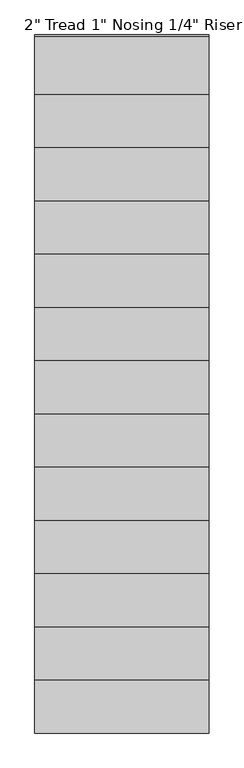
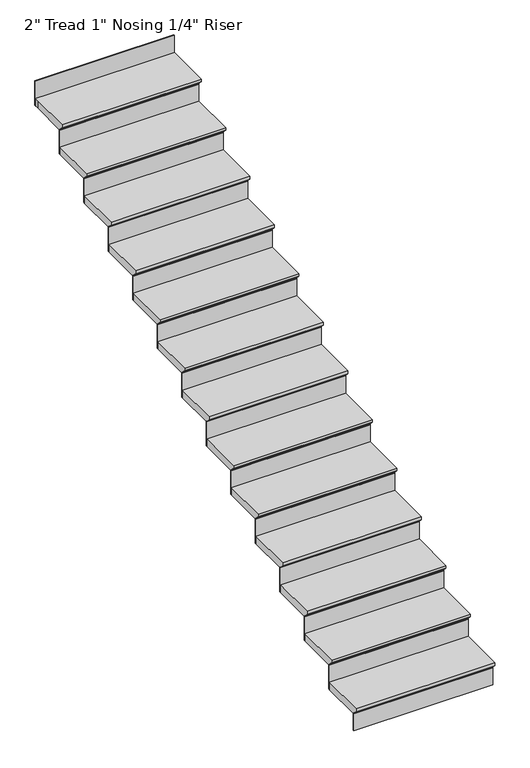
"""IFC4 building model written with IfcOpenShell, lengths in millimetres: stair flight geometry."""

from ifc_helpers import new_model, si_unit, origin, place, context, project, spatial, faceted_brep, source, transform, mapped, element, save


def stair_flight_c80e62dd(model_context):
    return source(origin(), model_context, "Body", "Brep", [
        faceted_brep([(-2703.0415084, -23154.3851539, 37576.9005799), (-2703.0415084, -23154.3851539, 37595.9505799), (-3617.4415084, -23154.3851539, 37595.9505799), (-3617.4415084, -23154.3851539, 37576.9005799), (-2703.0415084, -23128.9851539, 37551.5005799), (-3617.4415084, -23128.9851539, 37551.5005799), (-2703.0415084, -22849.5851539, 37595.9505799), (-3617.4415084, -22849.5851539, 37595.9505799), (-3617.4415084, -23128.9851539, 37545.1505799), (-3617.4415084, -22849.5851539, 37545.1505799), (-2703.0415084, -22849.5851539, 37545.1505799), (-2703.0415084, -23128.9851539, 37545.1505799)], [[[0, 1, 2, 3]], [[4, 0, 3, 5]], [[2, 1, 6, 7]], [[8, 9, 10, 11]], [[2, 7, 9, 8, 5, 3]], [[8, 11, 4, 5]], [[6, 1, 0, 4, 11, 10]], [[7, 6, 10, 9]]]),
        faceted_brep([(-2703.0415084, -23128.9851539, 37545.1505799), (-2703.0415084, -23128.9851539, 37426.6172466), (-2703.0415084, -23122.6351539, 37426.6172466), (-2703.0415084, -23122.6351539, 37545.1505799), (-3617.4415084, -23128.9851539, 37545.1505799), (-3617.4415084, -23122.6351539, 37545.1505799), (-3617.4415084, -23122.6351539, 37426.6172466), (-3617.4415084, -23128.9851539, 37426.6172466)], [[[0, 1, 2, 3]], [[4, 5, 6, 7]], [[1, 0, 4, 7]], [[2, 1, 7, 6]], [[3, 2, 6, 5]], [[0, 3, 5, 4]]]),
        faceted_brep([(-2703.0415084, -22849.5851539, 37714.4839133), (-2703.0415084, -22849.5851539, 37545.1505799), (-2703.0415084, -22843.2351539, 37545.1505799), (-2703.0415084, -22843.2351539, 37714.4839133), (-3617.4415084, -22849.5851539, 37714.4839133), (-3617.4415084, -22843.2351539, 37714.4839133), (-3617.4415084, -22843.2351539, 37545.1505799), (-3617.4415084, -22849.5851539, 37545.1505799)], [[[0, 1, 2, 3]], [[4, 5, 6, 7]], [[1, 0, 4, 7]], [[2, 1, 7, 6]], [[3, 2, 6, 5]], [[0, 3, 5, 4]]]),
        faceted_brep([(-3617.4415084, -22874.9851539, 37765.2839133), (-2703.0415084, -22874.9851539, 37765.2839133), (-2703.0415084, -22570.1851539, 37765.2839133), (-3617.4415084, -22570.1851539, 37765.2839133), (-3617.4415084, -22849.5851539, 37714.4839133), (-3617.4415084, -22570.1851539, 37714.4839133), (-2703.0415084, -22570.1851539, 37714.4839133), (-2703.0415084, -22849.5851539, 37714.4839133), (-3617.4415084, -22849.5851539, 37720.8339133), (-3617.4415084, -22874.9851539, 37746.2339133), (-2703.0415084, -22849.5851539, 37720.8339133), (-2703.0415084, -22874.9851539, 37746.2339133)], [[[0, 1, 2, 3]], [[4, 5, 6, 7]], [[0, 3, 5, 4, 8, 9]], [[4, 7, 10, 8]], [[2, 1, 11, 10, 7, 6]], [[3, 2, 6, 5]], [[11, 1, 0, 9]], [[10, 11, 9, 8]]]),
        faceted_brep([(-2703.0415084, -22570.1851539, 37883.8172466), (-2703.0415084, -22570.1851539, 37714.4839133), (-2703.0415084, -22563.8351539, 37714.4839133), (-2703.0415084, -22563.8351539, 37883.8172466), (-3617.4415084, -22570.1851539, 37883.8172466), (-3617.4415084, -22563.8351539, 37883.8172466), (-3617.4415084, -22563.8351539, 37714.4839133), (-3617.4415084, -22570.1851539, 37714.4839133)], [[[0, 1, 2, 3]], [[4, 5, 6, 7]], [[1, 0, 4, 7]], [[2, 1, 7, 6]], [[3, 2, 6, 5]], [[0, 3, 5, 4]]]),
        faceted_brep([(-3617.4415084, -22595.5851539, 37934.6172466), (-2703.0415084, -22595.5851539, 37934.6172466), (-2703.0415084, -22290.7851539, 37934.6172466), (-3617.4415084, -22290.7851539, 37934.6172466), (-3617.4415084, -22570.1851539, 37883.8172466), (-3617.4415084, -22290.7851539, 37883.8172466), (-2703.0415084, -22290.7851539, 37883.8172466), (-2703.0415084, -22570.1851539, 37883.8172466), (-3617.4415084, -22570.1851539, 37890.1672466), (-3617.4415084, -22595.5851539, 37915.5672466), (-2703.0415084, -22570.1851539, 37890.1672466), (-2703.0415084, -22595.5851539, 37915.5672466)], [[[0, 1, 2, 3]], [[4, 5, 6, 7]], [[0, 3, 5, 4, 8, 9]], [[4, 7, 10, 8]], [[2, 1, 11, 10, 7, 6]], [[3, 2, 6, 5]], [[11, 1, 0, 9]], [[10, 11, 9, 8]]]),
        faceted_brep([(-2703.0415084, -22290.7851539, 38053.1505799), (-2703.0415084, -22290.7851539, 37883.8172466), (-2703.0415084, -22284.4351539, 37883.8172466), (-2703.0415084, -22284.4351539, 38053.1505799), (-3617.4415084, -22290.7851539, 38053.1505799), (-3617.4415084, -22284.4351539, 38053.1505799), (-3617.4415084, -22284.4351539, 37883.8172466), (-3617.4415084, -22290.7851539, 37883.8172466)], [[[0, 1, 2, 3]], [[4, 5, 6, 7]], [[1, 0, 4, 7]], [[2, 1, 7, 6]], [[3, 2, 6, 5]], [[0, 3, 5, 4]]]),
        faceted_brep([(-3617.4415084, -22316.1851539, 38103.9505799), (-2703.0415084, -22316.1851539, 38103.9505799), (-2703.0415084, -22011.3851539, 38103.9505799), (-3617.4415084, -22011.3851539, 38103.9505799), (-3617.4415084, -22290.7851539, 38053.1505799), (-3617.4415084, -22011.3851539, 38053.1505799), (-2703.0415084, -22011.3851539, 38053.1505799), (-2703.0415084, -22290.7851539, 38053.1505799), (-3617.4415084, -22290.7851539, 38059.5005799), (-3617.4415084, -22316.1851539, 38084.9005799), (-2703.0415084, -22290.7851539, 38059.5005799), (-2703.0415084, -22316.1851539, 38084.9005799)], [[[0, 1, 2, 3]], [[4, 5, 6, 7]], [[0, 3, 5, 4, 8, 9]], [[4, 7, 10, 8]], [[2, 1, 11, 10, 7, 6]], [[3, 2, 6, 5]], [[11, 1, 0, 9]], [[10, 11, 9, 8]]]),
        faceted_brep([(-2703.0415084, -22011.3851539, 38222.4839133), (-2703.0415084, -22011.3851539, 38053.1505799), (-2703.0415084, -22005.0351539, 38053.1505799), (-2703.0415084, -22005.0351539, 38222.4839133), (-3617.4415084, -22011.3851539, 38222.4839133), (-3617.4415084, -22005.0351539, 38222.4839133), (-3617.4415084, -22005.0351539, 38053.1505799), (-3617.4415084, -22011.3851539, 38053.1505799)], [[[0, 1, 2, 3]], [[4, 5, 6, 7]], [[1, 0, 4, 7]], [[2, 1, 7, 6]], [[3, 2, 6, 5]], [[0, 3, 5, 4]]]),
        faceted_brep([(-3617.4415084, -22036.7851539, 38273.2839133), (-2703.0415084, -22036.7851539, 38273.2839133), (-2703.0415084, -21731.9851539, 38273.2839133), (-3617.4415084, -21731.9851539, 38273.2839133), (-3617.4415084, -22011.3851539, 38222.4839133), (-3617.4415084, -21731.9851539, 38222.4839133), (-2703.0415084, -21731.9851539, 38222.4839133), (-2703.0415084, -22011.3851539, 38222.4839133), (-3617.4415084, -22011.3851539, 38228.8339133), (-3617.4415084, -22036.7851539, 38254.2339133), (-2703.0415084, -22011.3851539, 38228.8339133), (-2703.0415084, -22036.7851539, 38254.2339133)], [[[0, 1, 2, 3]], [[4, 5, 6, 7]], [[0, 3, 5, 4, 8, 9]], [[4, 7, 10, 8]], [[2, 1, 11, 10, 7, 6]], [[3, 2, 6, 5]], [[11, 1, 0, 9]], [[10, 11, 9, 8]]]),
        faceted_brep([(-2703.0415084, -21731.9851539, 38391.8172466), (-2703.0415084, -21731.9851539, 38222.4839133), (-2703.0415084, -21725.6351539, 38222.4839133), (-2703.0415084, -21725.6351539, 38391.8172466), (-3617.4415084, -21731.9851539, 38391.8172466), (-3617.4415084, -21725.6351539, 38391.8172466), (-3617.4415084, -21725.6351539, 38222.4839133), (-3617.4415084, -21731.9851539, 38222.4839133)], [[[0, 1, 2, 3]], [[4, 5, 6, 7]], [[1, 0, 4, 7]], [[2, 1, 7, 6]], [[3, 2, 6, 5]], [[0, 3, 5, 4]]]),
        faceted_brep([(-3617.4415084, -21757.3851539, 38442.6172466), (-2703.0415084, -21757.3851539, 38442.6172466), (-2703.0415084, -21452.5851539, 38442.6172466), (-3617.4415084, -21452.5851539, 38442.6172466), (-3617.4415084, -21731.9851539, 38391.8172466), (-3617.4415084, -21452.5851539, 38391.8172466), (-2703.0415084, -21452.5851539, 38391.8172466), (-2703.0415084, -21731.9851539, 38391.8172466), (-3617.4415084, -21731.9851539, 38398.1672466), (-3617.4415084, -21757.3851539, 38423.5672466), (-2703.0415084, -21731.9851539, 38398.1672466), (-2703.0415084, -21757.3851539, 38423.5672466)], [[[0, 1, 2, 3]], [[4, 5, 6, 7]], [[0, 3, 5, 4, 8, 9]], [[4, 7, 10, 8]], [[2, 1, 11, 10, 7, 6]], [[3, 2, 6, 5]], [[11, 1, 0, 9]], [[10, 11, 9, 8]]]),
        faceted_brep([(-2703.0415084, -21452.5851539, 38561.1505799), (-2703.0415084, -21452.5851539, 38391.8172466), (-2703.0415084, -21446.2351539, 38391.8172466), (-2703.0415084, -21446.2351539, 38561.1505799), (-3617.4415084, -21452.5851539, 38561.1505799), (-3617.4415084, -21446.2351539, 38561.1505799), (-3617.4415084, -21446.2351539, 38391.8172466), (-3617.4415084, -21452.5851539, 38391.8172466)], [[[0, 1, 2, 3]], [[4, 5, 6, 7]], [[1, 0, 4, 7]], [[2, 1, 7, 6]], [[3, 2, 6, 5]], [[0, 3, 5, 4]]]),
        faceted_brep([(-3617.4415084, -21477.9851539, 38611.9505799), (-2703.0415084, -21477.9851539, 38611.9505799), (-2703.0415084, -21173.1851539, 38611.9505799), (-3617.4415084, -21173.1851539, 38611.9505799), (-3617.4415084, -21452.5851539, 38561.1505799), (-3617.4415084, -21173.1851539, 38561.1505799), (-2703.0415084, -21173.1851539, 38561.1505799), (-2703.0415084, -21452.5851539, 38561.1505799), (-3617.4415084, -21452.5851539, 38567.5005799), (-3617.4415084, -21477.9851539, 38592.9005799), (-2703.0415084, -21452.5851539, 38567.5005799), (-2703.0415084, -21477.9851539, 38592.9005799)], [[[0, 1, 2, 3]], [[4, 5, 6, 7]], [[0, 3, 5, 4, 8, 9]], [[4, 7, 10, 8]], [[2, 1, 11, 10, 7, 6]], [[3, 2, 6, 5]], [[11, 1, 0, 9]], [[10, 11, 9, 8]]]),
        faceted_brep([(-2703.0415084, -21173.1851539, 38730.4839133), (-2703.0415084, -21173.1851539, 38561.1505799), (-2703.0415084, -21166.8351539, 38561.1505799), (-2703.0415084, -21166.8351539, 38730.4839133), (-3617.4415084, -21173.1851539, 38730.4839133), (-3617.4415084, -21166.8351539, 38730.4839133), (-3617.4415084, -21166.8351539, 38561.1505799), (-3617.4415084, -21173.1851539, 38561.1505799)], [[[0, 1, 2, 3]], [[4, 5, 6, 7]], [[1, 0, 4, 7]], [[2, 1, 7, 6]], [[3, 2, 6, 5]], [[0, 3, 5, 4]]]),
        faceted_brep([(-3617.4415084, -21198.5851539, 38781.2839133), (-2703.0415084, -21198.5851539, 38781.2839133), (-2703.0415084, -20893.7851539, 38781.2839133), (-3617.4415084, -20893.7851539, 38781.2839133), (-3617.4415084, -21173.1851539, 38730.4839133), (-3617.4415084, -20893.7851539, 38730.4839133), (-2703.0415084, -20893.7851539, 38730.4839133), (-2703.0415084, -21173.1851539, 38730.4839133), (-3617.4415084, -21173.1851539, 38736.8339133), (-3617.4415084, -21198.5851539, 38762.2339133), (-2703.0415084, -21173.1851539, 38736.8339133), (-2703.0415084, -21198.5851539, 38762.2339133)], [[[0, 1, 2, 3]], [[4, 5, 6, 7]], [[0, 3, 5, 4, 8, 9]], [[4, 7, 10, 8]], [[2, 1, 11, 10, 7, 6]], [[3, 2, 6, 5]], [[11, 1, 0, 9]], [[10, 11, 9, 8]]]),
        faceted_brep([(-2703.0415084, -20893.7851539, 38899.8172466), (-2703.0415084, -20893.7851539, 38730.4839133), (-2703.0415084, -20887.4351539, 38730.4839133), (-2703.0415084, -20887.4351539, 38899.8172466), (-3617.4415084, -20893.7851539, 38899.8172466), (-3617.4415084, -20887.4351539, 38899.8172466), (-3617.4415084, -20887.4351539, 38730.4839133), (-3617.4415084, -20893.7851539, 38730.4839133)], [[[0, 1, 2, 3]], [[4, 5, 6, 7]], [[1, 0, 4, 7]], [[2, 1, 7, 6]], [[3, 2, 6, 5]], [[0, 3, 5, 4]]]),
        faceted_brep([(-3617.4415084, -20919.1851539, 38950.6172466), (-2703.0415084, -20919.1851539, 38950.6172466), (-2703.0415084, -20614.3851539, 38950.6172466), (-3617.4415084, -20614.3851539, 38950.6172466), (-3617.4415084, -20893.7851539, 38899.8172466), (-3617.4415084, -20614.3851539, 38899.8172466), (-2703.0415084, -20614.3851539, 38899.8172466), (-2703.0415084, -20893.7851539, 38899.8172466), (-3617.4415084, -20893.7851539, 38906.1672466), (-3617.4415084, -20919.1851539, 38931.5672466), (-2703.0415084, -20893.7851539, 38906.1672466), (-2703.0415084, -20919.1851539, 38931.5672466)], [[[0, 1, 2, 3]], [[4, 5, 6, 7]], [[0, 3, 5, 4, 8, 9]], [[4, 7, 10, 8]], [[2, 1, 11, 10, 7, 6]], [[3, 2, 6, 5]], [[11, 1, 0, 9]], [[10, 11, 9, 8]]]),
        faceted_brep([(-2703.0415084, -20614.3851539, 39069.1505799), (-2703.0415084, -20614.3851539, 38899.8172466), (-2703.0415084, -20608.0351539, 38899.8172466), (-2703.0415084, -20608.0351539, 39069.1505799), (-3617.4415084, -20614.3851539, 39069.1505799), (-3617.4415084, -20608.0351539, 39069.1505799), (-3617.4415084, -20608.0351539, 38899.8172466), (-3617.4415084, -20614.3851539, 38899.8172466)], [[[0, 1, 2, 3]], [[4, 5, 6, 7]], [[1, 0, 4, 7]], [[2, 1, 7, 6]], [[3, 2, 6, 5]], [[0, 3, 5, 4]]]),
        faceted_brep([(-3617.4415084, -20639.7851539, 39119.9505799), (-2703.0415084, -20639.7851539, 39119.9505799), (-2703.0415084, -20334.9851539, 39119.9505799), (-3617.4415084, -20334.9851539, 39119.9505799), (-3617.4415084, -20614.3851539, 39069.1505799), (-3617.4415084, -20334.9851539, 39069.1505799), (-2703.0415084, -20334.9851539, 39069.1505799), (-2703.0415084, -20614.3851539, 39069.1505799), (-3617.4415084, -20614.3851539, 39075.5005799), (-3617.4415084, -20639.7851539, 39100.9005799), (-2703.0415084, -20614.3851539, 39075.5005799), (-2703.0415084, -20639.7851539, 39100.9005799)], [[[0, 1, 2, 3]], [[4, 5, 6, 7]], [[0, 3, 5, 4, 8, 9]], [[4, 7, 10, 8]], [[2, 1, 11, 10, 7, 6]], [[3, 2, 6, 5]], [[11, 1, 0, 9]], [[10, 11, 9, 8]]]),
        faceted_brep([(-2703.0415084, -20334.9851539, 39238.4839133), (-2703.0415084, -20334.9851539, 39069.1505799), (-2703.0415084, -20328.6351539, 39069.1505799), (-2703.0415084, -20328.6351539, 39238.4839133), (-3617.4415084, -20334.9851539, 39238.4839133), (-3617.4415084, -20328.6351539, 39238.4839133), (-3617.4415084, -20328.6351539, 39069.1505799), (-3617.4415084, -20334.9851539, 39069.1505799)], [[[0, 1, 2, 3]], [[4, 5, 6, 7]], [[1, 0, 4, 7]], [[2, 1, 7, 6]], [[3, 2, 6, 5]], [[0, 3, 5, 4]]]),
        faceted_brep([(-3617.4415084, -20360.3851539, 39289.2839133), (-2703.0415084, -20360.3851539, 39289.2839133), (-2703.0415084, -20055.5851539, 39289.2839133), (-3617.4415084, -20055.5851539, 39289.2839133), (-3617.4415084, -20334.9851539, 39238.4839133), (-3617.4415084, -20055.5851539, 39238.4839133), (-2703.0415084, -20055.5851539, 39238.4839133), (-2703.0415084, -20334.9851539, 39238.4839133), (-3617.4415084, -20334.9851539, 39244.8339133), (-3617.4415084, -20360.3851539, 39270.2339133), (-2703.0415084, -20334.9851539, 39244.8339133), (-2703.0415084, -20360.3851539, 39270.2339133)], [[[0, 1, 2, 3]], [[4, 5, 6, 7]], [[0, 3, 5, 4, 8, 9]], [[4, 7, 10, 8]], [[2, 1, 11, 10, 7, 6]], [[3, 2, 6, 5]], [[11, 1, 0, 9]], [[10, 11, 9, 8]]]),
        faceted_brep([(-2703.0415084, -20055.5851539, 39407.8172466), (-2703.0415084, -20055.5851539, 39238.4839133), (-2703.0415084, -20049.2351539, 39238.4839133), (-2703.0415084, -20049.2351539, 39407.8172466), (-3617.4415084, -20055.5851539, 39407.8172466), (-3617.4415084, -20049.2351539, 39407.8172466), (-3617.4415084, -20049.2351539, 39238.4839133), (-3617.4415084, -20055.5851539, 39238.4839133)], [[[0, 1, 2, 3]], [[4, 5, 6, 7]], [[1, 0, 4, 7]], [[2, 1, 7, 6]], [[3, 2, 6, 5]], [[0, 3, 5, 4]]]),
        faceted_brep([(-3617.4415084, -20080.9851539, 39458.6172466), (-2703.0415084, -20080.9851539, 39458.6172466), (-2703.0415084, -19776.1851539, 39458.6172466), (-3617.4415084, -19776.1851539, 39458.6172466), (-3617.4415084, -20055.5851539, 39407.8172466), (-3617.4415084, -19776.1851539, 39407.8172466), (-2703.0415084, -19776.1851539, 39407.8172466), (-2703.0415084, -20055.5851539, 39407.8172466), (-3617.4415084, -20055.5851539, 39414.1672466), (-3617.4415084, -20080.9851539, 39439.5672466), (-2703.0415084, -20055.5851539, 39414.1672466), (-2703.0415084, -20080.9851539, 39439.5672466)], [[[0, 1, 2, 3]], [[4, 5, 6, 7]], [[0, 3, 5, 4, 8, 9]], [[4, 7, 10, 8]], [[2, 1, 11, 10, 7, 6]], [[3, 2, 6, 5]], [[11, 1, 0, 9]], [[10, 11, 9, 8]]]),
        faceted_brep([(-2703.0415084, -19496.7851539, 39746.4839133), (-2703.0415084, -19496.7851539, 39577.1505799), (-2703.0415084, -19490.4351539, 39577.1505799), (-2703.0415084, -19490.4351539, 39746.4839133), (-3617.4415084, -19496.7851539, 39746.4839133), (-3617.4415084, -19490.4351539, 39746.4839133), (-3617.4415084, -19490.4351539, 39577.1505799), (-3617.4415084, -19496.7851539, 39577.1505799)], [[[0, 1, 2, 3]], [[4, 5, 6, 7]], [[1, 0, 4, 7]], [[2, 1, 7, 6]], [[3, 2, 6, 5]], [[0, 3, 5, 4]]]),
        faceted_brep([(-2703.0415084, -19776.1851539, 39577.1505799), (-2703.0415084, -19776.1851539, 39407.8172466), (-2703.0415084, -19769.8351539, 39407.8172466), (-2703.0415084, -19769.8351539, 39577.1505799), (-3617.4415084, -19776.1851539, 39577.1505799), (-3617.4415084, -19769.8351539, 39577.1505799), (-3617.4415084, -19769.8351539, 39407.8172466), (-3617.4415084, -19776.1851539, 39407.8172466)], [[[0, 1, 2, 3]], [[4, 5, 6, 7]], [[1, 0, 4, 7]], [[2, 1, 7, 6]], [[3, 2, 6, 5]], [[0, 3, 5, 4]]]),
        faceted_brep([(-3617.4415084, -19496.7851539, 39627.9505799), (-3617.4415084, -19522.1851539, 39627.9505799), (-3617.4415084, -19801.5851539, 39627.9505799), (-2703.0415084, -19801.5851539, 39627.9505799), (-2703.0415084, -19496.7851539, 39627.9505799), (-3617.4415084, -19522.1851539, 39577.1505799), (-3617.4415084, -19496.7851539, 39577.1505799), (-2703.0415084, -19496.7851539, 39577.1505799), (-2703.0415084, -19776.1851539, 39577.1505799), (-3617.4415084, -19776.1851539, 39577.1505799), (-3617.4415084, -19776.1851539, 39583.5005799), (-3617.4415084, -19801.5851539, 39608.9005799), (-2703.0415084, -19776.1851539, 39583.5005799), (-2703.0415084, -19801.5851539, 39608.9005799)], [[[0, 1, 2, 3, 4]], [[5, 6, 7, 8, 9]], [[1, 0, 6, 5]], [[2, 1, 5, 9, 10, 11]], [[9, 8, 12, 10]], [[4, 3, 13, 12, 8, 7]], [[0, 4, 7, 6]], [[13, 3, 2, 11]], [[12, 13, 11, 10]]]),
    ])


if __name__ == "__main__":
    model = new_model("IFC4")
    model_context = context("Model", 3, world=origin())
    ifc_project = project(units=[si_unit("LENGTHUNIT", "METRE", prefix="MILLI")], contexts=[model_context])
    site = spatial("IfcSite", under=ifc_project)
    building = spatial("IfcBuilding", under=site)
    placement = place(None, origin())
    stair_flight_shape = stair_flight_c80e62dd(model_context)
    element("IfcStairFlight", 1, ObjectType="2\" Tread 1\" Nosing 1/4\" Riser", at=placement, inside=building, context=model_context, shape_type="MappedRepresentation", body=[
        mapped(stair_flight_shape, transform((0.0, 0.0, 0.0), x_axis=(1.0, 0.0, 0.0), y_axis=(0.0, 1.0, 0.0), z_axis=(0.0, 0.0, 1.0))),
    ])
    save(model, "model.ifc")
